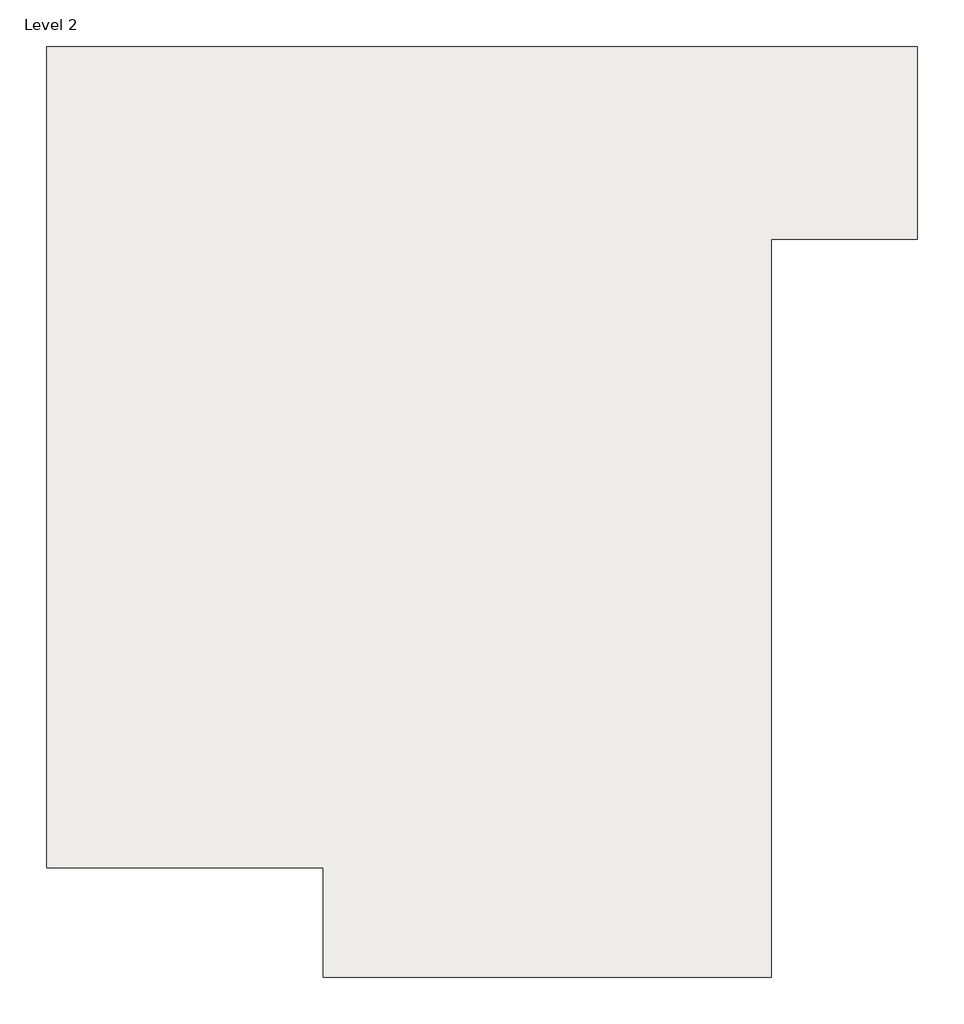
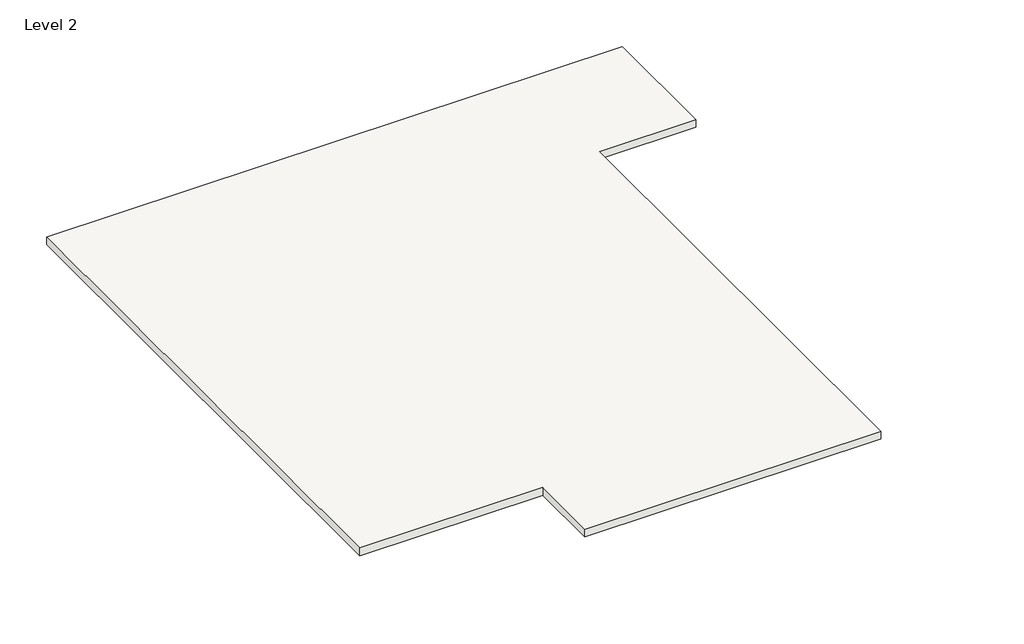
# One storey: 1 roof.
"""IFC4 building model written with IfcOpenShell, lengths in millimetres."""

from ifc_helpers import new_model, si_unit, frame, origin, place, context, project, spatial, polyline, outline, extrude, element, save

model = new_model("IFC4")

# Units and contexts
model_context = context("Model", 3, world=origin())
ifc_project = project(units=[si_unit("LENGTHUNIT", "METRE", prefix="MILLI")], contexts=[model_context])

# Site, building, storey
site = spatial("IfcSite", under=ifc_project)
building = spatial("IfcBuilding", under=site)
storey = spatial("IfcBuildingStorey", under=building, Name="Level 2", Elevation=3048.0)

# Roof
placement = place(None, origin())
element("IfcRoof", 1, ObjectType="Generic - 12\"", at=placement, inside=storey, context=model_context, shape_type="SweptSolid", body=[
    extrude(outline(polyline([(-6132.0415084, 8043.8940003), (4535.9584916, 8043.8940003), (4535.9584916, 5681.6935985), (2745.2584916, 5681.6935985), (2745.2584916, -3360.7064015), (-2741.1415084, -3360.7064015), (-2741.1415084, -2014.5064015), (-6132.0415084, -2014.5064015), (-6132.0415084, 8043.8940003)])), frame((0.0, 0.0, 3048.0), z_axis=(0.0, 0.0, 1.0), x_axis=(1.0, 0.0, 0.0)), (0.0, 0.0, 1.0), 152.4),
])

save(model, "model.ifc")

# Revit data of these elements
# Type "Generic - 12\""
#   Assembly Code = "B1020"
#   Layers, outside or top first: 0' - 6" no material (function 1)
# Element 1 (IfcRoof, "Generic - 12\"")
#   built-in parameter 1001705 = 10.5 (stored number, unit not read)
#   built-in parameter 1001710 = 33615
#   Phase Created = New Construction
#   Materials on its faces: "Default Roof", "Wood - Stained"
# Materials
#   "Default Roof": colour RGB 88 101 114, transparency 0, Cost = 0
#   "Wood - Stained": class "Wood", colour RGB 224 178 126, transparency 0, Cost = 0
